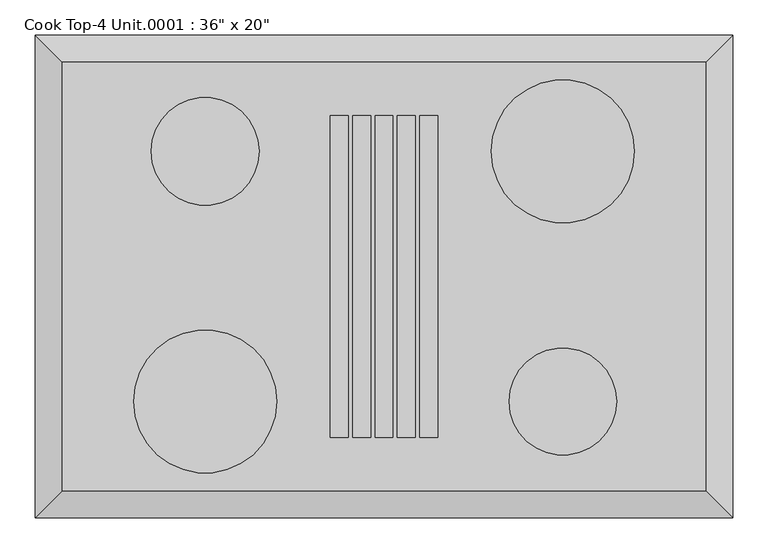
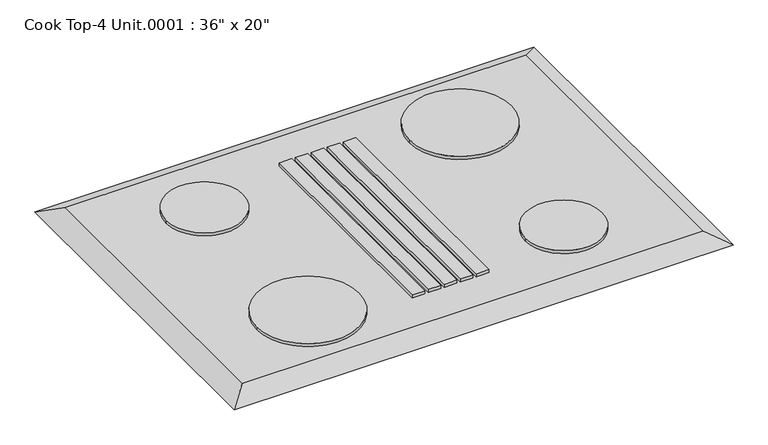
"""IFC4 building model written with IfcOpenShell, lengths in millimetres: proxy geometry."""

from ifc_helpers import new_model, si_unit, point, frame, frame_2d, origin, place, context, project, spatial, polyline, circle_curve, trimmed, segment, composite_curve, outline, extrude, faceted_brep, source, transform, mapped, element, save


def proxy_bb1e6e30(model_context):
    return source(origin(), model_context, "Body", "SolidModel", [
        extrude(outline(composite_curve([segment(trimmed(circle_curve(frame_2d((-254.0, 177.8)), 76.5869489), [point((-177.4130511, 177.8))], [point((-330.5869489, 177.8))], False, "CARTESIAN"), True, "CONTINUOUS"), segment(trimmed(circle_curve(frame_2d((-254.0, 177.8)), 76.5869489), [point((-330.5869489, 177.8))], [point((-177.4130511, 177.8))], False, "CARTESIAN"), True, "CONTINUOUS")], self_intersect=False)), frame((0.0, 0.0, 806.45), z_axis=(0.0, 0.0, 1.0), x_axis=(1.0, 0.0, 0.0)), (0.0, 0.0, 1.0), 6.35),
        extrude(outline(composite_curve([segment(trimmed(circle_curve(frame_2d((254.0, 177.8)), 101.6), [point((355.6, 177.8))], [point((152.4, 177.8))], False, "CARTESIAN"), True, "CONTINUOUS"), segment(trimmed(circle_curve(frame_2d((254.0, 177.8)), 101.6), [point((152.4, 177.8))], [point((355.6, 177.8))], False, "CARTESIAN"), True, "CONTINUOUS")], self_intersect=False)), frame((0.0, 0.0, 806.45), z_axis=(0.0, 0.0, 1.0), x_axis=(1.0, 0.0, 0.0)), (0.0, 0.0, 1.0), 6.35),
        extrude(outline(composite_curve([segment(trimmed(circle_curve(frame_2d((254.0, -177.8)), 76.2), [point((330.2, -177.8))], [point((177.8, -177.8))], False, "CARTESIAN"), True, "CONTINUOUS"), segment(trimmed(circle_curve(frame_2d((254.0, -177.8)), 76.2), [point((177.8, -177.8))], [point((330.2, -177.8))], False, "CARTESIAN"), True, "CONTINUOUS")], self_intersect=False)), frame((0.0, 0.0, 806.45), z_axis=(0.0, 0.0, 1.0), x_axis=(1.0, 0.0, 0.0)), (0.0, 0.0, 1.0), 6.35),
        extrude(outline(polyline([(-50.8, 228.6), (-50.8, -228.6), (-76.2, -228.6), (-76.2, 228.6), (-50.8, 228.6)])), frame((0.0, 0.0, 806.45), z_axis=(0.0, 0.0, 1.0), x_axis=(1.0, 0.0, 0.0)), (0.0, 0.0, 1.0), 6.35),
        extrude(outline(polyline([(-19.05, 228.6), (-19.05, -228.6), (-44.45, -228.6), (-44.45, 228.6), (-19.05, 228.6)])), frame((0.0, 0.0, 806.45), z_axis=(0.0, 0.0, 1.0), x_axis=(1.0, 0.0, 0.0)), (0.0, 0.0, 1.0), 6.35),
        extrude(outline(polyline([(12.7, 228.6), (12.7, -228.6), (-12.7, -228.6), (-12.7, 228.6), (12.7, 228.6)])), frame((0.0, 0.0, 806.45), z_axis=(0.0, 0.0, 1.0), x_axis=(1.0, 0.0, 0.0)), (0.0, 0.0, 1.0), 6.35),
        extrude(outline(polyline([(44.45, 228.6), (44.45, -228.6), (19.05, -228.6), (19.05, 228.6), (44.45, 228.6)])), frame((0.0, 0.0, 806.45), z_axis=(0.0, 0.0, 1.0), x_axis=(1.0, 0.0, 0.0)), (0.0, 0.0, 1.0), 6.35),
        extrude(outline(polyline([(76.2, 228.6), (76.2, -228.6), (50.8, -228.6), (50.8, 228.6), (76.2, 228.6)])), frame((0.0, 0.0, 806.45), z_axis=(0.0, 0.0, 1.0), x_axis=(1.0, 0.0, 0.0)), (0.0, 0.0, 1.0), 6.35),
        faceted_brep([(457.2, 304.8, 806.45), (-457.2, 304.8, 806.45), (-457.2, -304.8, 806.45), (457.2, -304.8, 806.45), (495.3, 342.9, 787.4), (495.3, -342.9, 787.4), (-495.3, -342.9, 787.4), (-495.3, 342.9, 787.4)], [[[0, 1, 2, 3]], [[4, 5, 6, 7]], [[4, 7, 1, 0]], [[7, 6, 2, 1]], [[6, 5, 3, 2]], [[5, 4, 0, 3]]]),
        extrude(outline(composite_curve([segment(trimmed(circle_curve(frame_2d((-254.0, -177.8)), 101.6), [point((-152.4, -177.8))], [point((-355.6, -177.8))], False, "CARTESIAN"), True, "CONTINUOUS"), segment(trimmed(circle_curve(frame_2d((-254.0, -177.8)), 101.6), [point((-355.6, -177.8))], [point((-152.4, -177.8))], False, "CARTESIAN"), True, "CONTINUOUS")], self_intersect=False)), frame((0.0, 0.0, 806.45), z_axis=(0.0, 0.0, 1.0), x_axis=(1.0, 0.0, 0.0)), (0.0, 0.0, 1.0), 6.35),
    ])


if __name__ == "__main__":
    model = new_model("IFC4")
    model_context = context("Model", 3, world=origin())
    ifc_project = project(units=[si_unit("LENGTHUNIT", "METRE", prefix="MILLI")], contexts=[model_context])
    site = spatial("IfcSite", under=ifc_project)
    building = spatial("IfcBuilding", under=site)
    placement = place(None, origin())
    proxy_shape = proxy_bb1e6e30(model_context)
    element("IfcBuildingElementProxy", 1, Name="Cook Top-4 Unit.0001 : 36\" x 20\"", ObjectType="Cook Top-4 Unit.0001 : 36\" x 20\"", at=placement, inside=building, context=model_context, shape_type="MappedRepresentation", body=[
        mapped(proxy_shape, transform((0.0, 0.0, 0.0), x_axis=(1.0, 0.0, 0.0), y_axis=(0.0, 1.0, 0.0), z_axis=(0.0, 0.0, 1.0))),
    ])
    save(model, "model.ifc")

# Revit data of these elements
# Type "Cook Top-4 Unit.0001 : 36\" x 20\""
#   Assembly Code = "E1090400"
#   Depth = 2' - 0"
#   Width = 3' - 0"
#   Burner Material = Steel, Chrome Plated
#   Cooktop Material = Steel, Polished
#   Default Elevation = 0
# Element 1 (IfcBuildingElementProxy, "Cook Top-4 Unit.0001 : 36\" x 20\"")
#   Materials on its faces: "Steel, Chrome Plated", "Steel, Polished"
# Materials
#   "Steel, Chrome Plated": class "Metal", colour RGB 17 17 17, transparency 0, Description = "Chromiuim plated steel", Cost = 0
#   "Steel, Polished": class "Metal", colour RGB 192 192 192, transparency 0, Description = "Polished steel", Cost = 0
